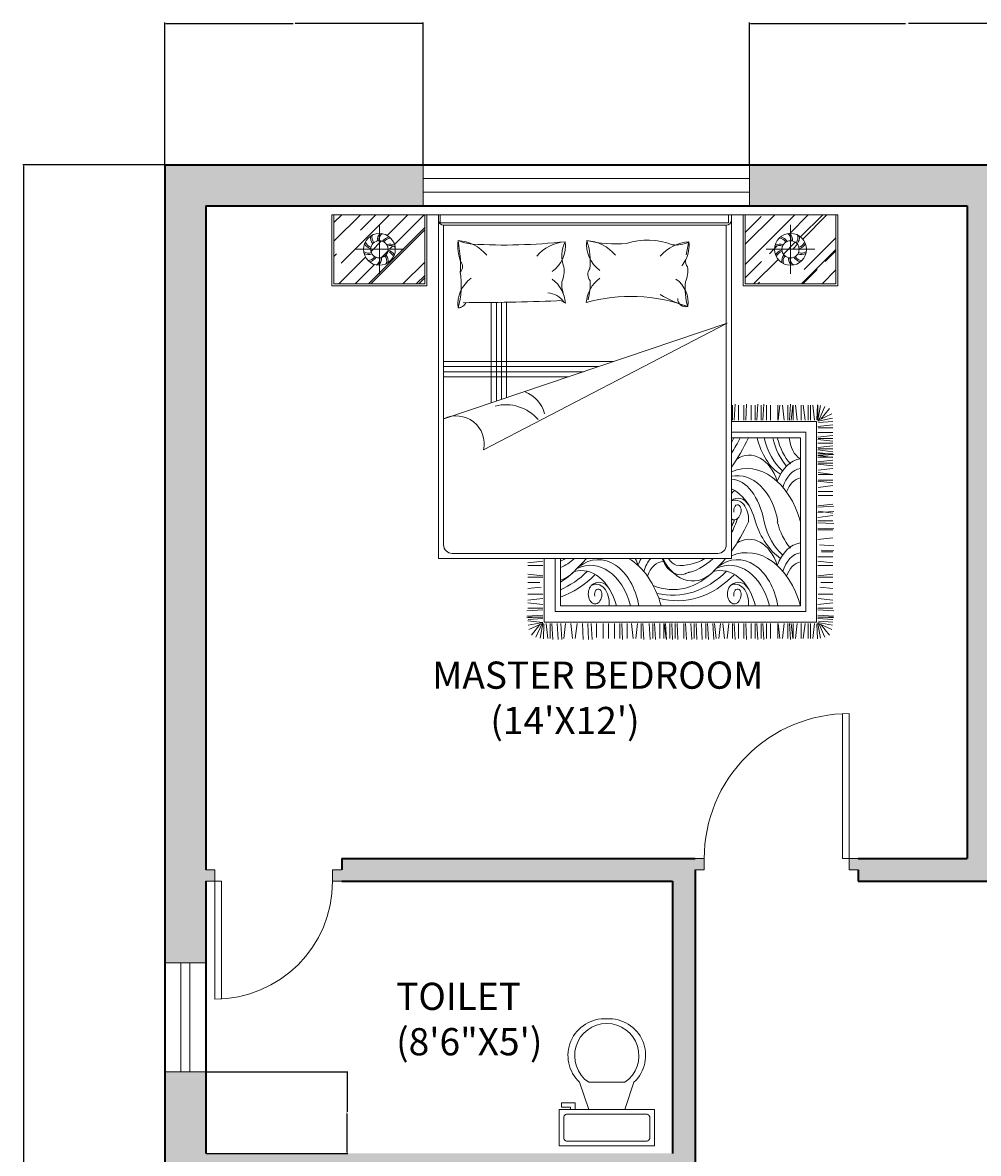
# Model space of a CAD drawing. Units: inches. Extents: x 2948 to 4025, y 2171 to 2966.
# Tile 3 of 6: x 2948 to 3159, y 2560 to 2809. Entities that reach past the tile are written whole.
import ezdxf

# ---------------------------------------------------------------- set-up
doc = ezdxf.new("R2010")
doc.units = ezdxf.units.IN
for name, color, linetype, lineweight in [('A-ANNO-DIMS', 2, 'Continuous', 18), ('A-AREA-IDEN', 7, 'Continuous', 18), ('A-DOOR', 3, 'Continuous', 18), ('A-FLOR-FIXT', 9, 'Continuous', 18), ('A-FURN', 8, 'Continuous', 18), ('A-GLAZ', 4, 'Continuous', 18), ('A-WALL', 7, 'Continuous', 35), ('A-WALL-PATT', 252, 'Continuous', 13)]:
    doc.layers.add(name, color=color, linetype=linetype, lineweight=lineweight)
doc.styles.get("Standard").update_dxf_attribs({"font": 'arial.ttf'})
doc.dimstyles.get("Standard").update_dxf_attribs({"dimtxt": 0.18, "dimasz": 0.18, "dimexe": 0.18, "dimexo": 0.0625, "dimgap": 0.09, "dimtad": 0, "dimtih": 1, "dimtoh": 1, "dimdec": 4, "dimzin": 0, "dimdsep": 46, "dimtxsty": 'Standard', "dimcen": 0.09, "dimadec": 0, "dimazin": 0, "dimtfac": 1, "dimtdec": 4, "dimtofl": 0, "dimtmove": 0, "dimatfit": 3, "dimfxl": 1, "dimtolj": 1, "dimtzin": 0, "dimarcsym": 0})

# ---------------------------------------------------------------- blocks, each defined once
blk = doc.blocks.new('A$C64B41DC1')
for p, q in [((0, 2.5079), (2.9903, 2.5079)), ((0, 2.0879), (0, 2.5079)), ((0.012, 2.4618), (0.0581, 2.5079)), ((0.012, 2.3515), (0.1684, 2.5079)), ((0.012, 2.0999), (0.012, 2.5079)), ((0.0543, 2.2213), (0.3409, 2.5079)), ((0.1689, 2.4179), (0.2589, 2.5079)), ((0.3265, 2.386), (0.4484, 2.5079)), ((0.3699, 2.3332), (0.5445, 2.5079)), ((0.548, 2.5079), (0.548, 2.0999)), ((0.56, 2.5079), (0.56, 2.0879)), ((0.6301, 2.5079), (0.6301, 0.4779)), ((0.6401, 2.461), (0.6401, 2.5079)), ((0.6401, 2.5079), (2.344, 2.5079)), ((2.344, 2.5079), (2.3601, 2.5079)), ((2.344, 2.5079), (2.344, 2.461)), ((2.3601, 2.5079), (2.3601, 2.4761)), ((2.3601, 0.4779), (2.3601, 2.5079)), ((2.4303, 2.5079), (2.4303, 2.0879)), ((2.4423, 2.5079), (2.4423, 2.0999)), ((2.4423, 2.3333), (2.6169, 2.5079)), ((2.4423, 2.2145), (2.7357, 2.5079)), ((2.4423, 2.404), (2.5354, 2.4971)), ((2.705, 2.398), (2.8149, 2.5079)), ((2.7691, 2.3772), (2.8998, 2.5079)), ((2.7819, 2.3646), (2.9252, 2.5079)), ((2.9783, 2.0999), (2.9783, 2.5079)), ((2.9903, 2.0879), (2.9903, 2.5079)), ((0.2157, 2.0999), (0.548, 2.4322)), ((0.2299, 2.0999), (0.548, 2.418)), ((0.2804, 2.1597), (0.2804, 2.4481)), ((2.344, 2.461), (0.6401, 2.461)), ((0.6601, 2.4461), (1.4951, 2.4461)), ((0.6601, 2.4461), (0.6601, 0.5579)), ((1.4951, 2.4461), (0.6697, 2.4461)), ((2.3301, 2.4461), (1.4951, 2.4461)), ((2.3301, 0.5579), (2.3301, 2.4461)), ((2.7099, 2.1597), (2.7099, 2.4481)), ((0.2311, 2.2906), (0.2937, 2.3532)), ((2.6674, 2.2756), (2.7382, 2.3464)), ((2.7914, 2.1846), (2.9783, 2.3715)), ((0.012, 2.261), (0.0275, 2.2765)), ((0.1362, 2.3039), (0.4246, 2.3039)), ((0.2905, 2.2539), (0.3304, 2.2938)), ((0.3405, 2.3039), (0.3605, 2.3238)), ((2.8541, 2.3039), (2.5657, 2.3039)), ((2.5849, 2.2779), (2.6158, 2.3088)), ((2.6158, 2.3088), (2.6313, 2.3243)), ((2.7249, 2.3076), (2.7512, 2.3339)), ((2.7746, 2.0999), (2.9783, 2.3036)), ((2.9144, 2.2312), (2.9783, 2.2951)), ((0.0404, 2.0999), (0.1982, 2.2578)), ((0.1365, 2.0999), (0.251, 2.2144)), ((0.4194, 2.0999), (0.548, 2.2285)), ((2.4423, 2.1353), (2.5382, 2.2312)), ((2.4918, 2.0999), (2.6366, 2.2447)), ((0.4986, 2.0999), (0.548, 2.1493)), ((2.7831, 2.0999), (2.8678, 2.1846)), ((2.8962, 2.0999), (2.9783, 2.182)), ((0.56, 2.0879), (0, 2.0879)), ((0.548, 2.0999), (0.012, 2.0999)), ((0.5127, 2.0999), (0.548, 2.1352)), ((2.4303, 2.0879), (2.9903, 2.0879)), ((2.4423, 2.0999), (2.9783, 2.0999)), ((2.5172, 2.0999), (2.5269, 2.1096)), ((0.9415, 1.9902), (0.9415, 1.3975)), ((0.9715, 1.9906), (0.9715, 1.4076)), ((1.0015, 1.991), (1.0015, 1.4177)), ((1.0315, 1.9916), (1.0315, 1.4279)), ((2.3349, 1.8678), (0.6613, 1.3029)), ((0.8956, 1.1191), (2.3349, 1.8678)), ((1.6636, 1.6412), (0.6601, 1.6412)), ((1.5748, 1.6112), (0.6601, 1.6112)), ((2.3665, 1.295), (2.3665, 1.3839)), ((2.377, 1.295), (2.3822, 1.3891)), ((2.4032, 1.295), (2.4032, 1.3839)), ((2.4346, 1.295), (2.4346, 1.3839)), ((2.4451, 1.295), (2.4503, 1.3891)), ((2.4774, 1.2957), (2.4774, 1.3837)), ((2.5, 1.295), (2.5, 1.3839)), ((2.5105, 1.295), (2.5157, 1.3891)), ((2.5367, 1.295), (2.5367, 1.3839)), ((2.5471, 1.295), (2.5524, 1.3891)), ((2.5681, 1.295), (2.5681, 1.3839)), ((2.5918, 1.295), (2.5918, 1.3839)), ((2.6346, 1.2957), (2.6346, 1.3837)), ((2.6362, 1.2957), (2.6467, 1.3839)), ((2.6729, 1.295), (2.6624, 1.3839)), ((2.6938, 1.295), (2.6938, 1.3839)), ((2.7043, 1.295), (2.7095, 1.3891)), ((2.7127, 1.2957), (2.7232, 1.3839)), ((2.7253, 1.295), (2.7253, 1.3839)), ((2.7494, 1.295), (2.7389, 1.3839)), ((2.7718, 1.295), (2.7718, 1.3839)), ((2.7959, 1.295), (2.7854, 1.3839)), ((2.8146, 1.2957), (2.8146, 1.3837)), ((2.8146, 1.2957), (2.8146, 1.3837)), ((2.8282, 1.295), (2.8282, 1.3839)), ((2.8282, 1.295), (2.8282, 1.3839)), ((2.8523, 1.295), (2.8418, 1.3839)), ((2.8523, 1.295), (2.8418, 1.3839)), ((2.8653, 1.2966), (2.8688, 1.3861)), ((2.8711, 1.2957), (2.8711, 1.3837)), ((2.8711, 1.2957), (2.8875, 1.3822)), ((2.8765, 1.2958), (2.9132, 1.3758)), ((2.8893, 1.3011), (2.9394, 1.3636)), ((2.3601, 1.2873), (2.8639, 1.2873)), ((2.8639, 1.2873), (2.8639, 0.1018)), ((2.8713, 1.2927), (2.954, 1.3315)), ((2.8717, 1.2884), (2.9588, 1.3058)), ((2.8744, 1.2817), (2.9603, 1.2869)), ((2.3601, 1.2233), (2.7999, 1.2233)), ((2.7999, 1.2233), (2.7999, 0.1658)), ((2.8716, 1.2565), (2.9605, 1.2669)), ((2.8716, 1.2212), (2.9605, 1.2212)), ((2.8716, 1.1947), (2.9605, 1.2052)), ((2.8723, 1.2489), (2.9603, 1.2489)), ((2.3601, 1.1913), (2.7679, 1.1912)), ((2.7679, 1.1912), (2.7679, 0.1978)), ((2.8716, 1.181), (2.9605, 1.1705)), ((2.8716, 1.1595), (2.9605, 1.1595)), ((2.8716, 1.133), (2.9605, 1.1435)), ((2.8723, 1.1872), (2.9603, 1.1872)), ((2.8716, 1.1193), (2.9605, 1.1088)), ((2.8716, 1.1035), (2.9605, 1.093)), ((2.8716, 1.0965), (2.9605, 1.0965)), ((2.8716, 1.086), (2.9657, 1.0913)), ((2.8716, 1.0756), (2.9605, 1.0756)), ((2.8723, 1.1255), (2.9603, 1.1255)), ((2.8723, 1.0858), (2.9605, 1.0753)), ((2.8716, 1.0491), (2.9605, 1.0596)), ((2.8716, 1.0354), (2.9605, 1.0249)), ((2.8723, 1.0416), (2.9603, 1.0416)), ((2.8723, 0.9987), (2.9605, 1.0092)), ((2.8723, 0.985), (2.9605, 0.9745)), ((2.8723, 0.9735), (2.9603, 0.9735)), ((2.8723, 0.9408), (2.9603, 0.9408)), ((2.8716, 0.9346), (2.9605, 0.9241)), ((2.8723, 0.8979), (2.9605, 0.9084)), ((2.8723, 0.8726), (2.9603, 0.8726)), ((2.8723, 0.8505), (2.9603, 0.8505)), ((2.8716, 0.7885), (2.9605, 0.799)), ((2.8716, 0.7818), (2.9657, 0.787)), ((2.8716, 0.7503), (2.9657, 0.7556)), ((2.8723, 0.7571), (2.9605, 0.7466)), ((2.8716, 0.7204), (2.9605, 0.7309)), ((2.8716, 0.6995), (2.9605, 0.6995)), ((2.8716, 0.689), (2.9657, 0.6838)), ((2.8716, 0.6576), (2.9657, 0.6523)), ((2.8716, 0.6471), (2.9605, 0.6471)), ((2.8716, 0.5903), (2.9605, 0.6007)), ((2.882, 0.5582), (2.9657, 0.5536)), ((0.6301, 0.4779), (2.3601, 0.4779)), ((0.7101, 0.5079), (2.2801, 0.5079)), ((1.2542, 0.1018), (1.2542, 0.4779)), ((1.3182, 0.1658), (1.3182, 0.4779)), ((1.3502, 0.1978), (1.3502, 0.4779)), ((2.8716, 0.4877), (2.9603, 0.4877)), ((2.8909, 0.5263), (2.9657, 0.5222)), ((2.8928, 0.5169), (2.9605, 0.5169)), ((1.2465, 0.4625), (1.1576, 0.452)), ((1.2465, 0.4365), (1.1577, 0.4365)), ((2.8716, 0.4625), (2.9605, 0.452)), ((2.8716, 0.4365), (2.9603, 0.4365)), ((1.2465, 0.3746), (1.1576, 0.3851)), ((1.2465, 0.3684), (1.1577, 0.3684)), ((1.2285, 0.3357), (1.1577, 0.3357)), ((2.8716, 0.3746), (2.9605, 0.3851)), ((2.8716, 0.3684), (2.9603, 0.3684)), ((2.8896, 0.3357), (2.9603, 0.3357)), ((1.2355, 0.3092), (1.1576, 0.3)), ((1.2457, 0.2676), (1.1577, 0.2676)), ((2.8723, 0.2676), (2.9603, 0.2676)), ((2.8826, 0.3092), (2.9605, 0.3)), ((1.2457, 0.2423), (1.1576, 0.2319)), ((1.2465, 0.2057), (1.1576, 0.2161)), ((2.8716, 0.2057), (2.9605, 0.2161)), ((2.8723, 0.2423), (2.9605, 0.2319)), ((1.2465, 0.1742), (1.1524, 0.169)), ((1.2465, 0.1428), (1.1524, 0.1376)), ((1.2465, 0.1847), (1.1576, 0.1847)), ((2.7999, 0.1658), (1.3182, 0.1658)), ((2.7679, 0.1978), (1.3502, 0.1978)), ((2.8716, 0.1847), (2.9605, 0.1847)), ((2.8716, 0.1742), (2.9657, 0.169)), ((2.8716, 0.1428), (2.9657, 0.1376)), ((1.2465, 0.1334), (1.1524, 0.1281)), ((1.2465, 0.1323), (1.1576, 0.1323)), ((1.2465, 0.1323), (1.1576, 0.1323)), ((1.2465, 0.1), (1.1576, 0.1105)), ((1.2465, 0.1229), (1.1588, 0.1168)), ((1.2464, 0.1007), (1.1592, 0.0833)), ((1.2468, 0.0964), (1.1641, 0.0576)), ((1.2288, 0.088), (1.1787, 0.0255)), ((1.2415, 0.0933), (1.2049, 0.0133)), ((1.247, 0.0934), (1.2306, 0.0069)), ((1.2527, 0.0925), (1.2493, 0.003)), ((2.8639, 0.1018), (1.2542, 0.1018)), ((1.2658, 0.0941), (1.2762, 0.0052)), ((1.2899, 0.0941), (1.2899, 0.0052)), ((1.2999, 0.0941), (1.3051, 0)), ((1.3313, 0.0941), (1.3365, 0)), ((1.3523, 0.0941), (1.3575, 0)), ((1.3804, 0.0941), (1.3699, 0.0052)), ((1.4119, 0.0934), (1.4223, 0.0052)), ((1.4485, 0.0941), (1.438, 0.0052)), ((1.48, 0.0941), (1.4852, 0)), ((1.5114, 0.0941), (1.5166, 0)), ((1.5323, 0.0941), (1.5376, 0)), ((1.5638, 0.0941), (1.5638, 0.0105)), ((1.6021, 0.0941), (1.6021, 0.0052)), ((1.6336, 0.0941), (1.6336, 0.0052)), ((1.6702, 0.0941), (1.6702, 0.0052)), ((1.7017, 0.0941), (1.7017, 0.0052)), ((1.7122, 0.0941), (1.7174, 0)), ((1.7445, 0.0934), (1.7445, 0.0054)), ((1.7698, 0.0934), (1.7803, 0.0052)), ((1.8065, 0.0941), (1.796, 0.0052)), ((1.8274, 0.0941), (1.8274, 0.0052)), ((1.8379, 0.0941), (1.8431, 0)), ((1.8746, 0.0941), (1.8798, 0)), ((1.8955, 0.0941), (1.8955, 0.0052)), ((1.906, 0.0941), (1.9113, 0)), ((1.9384, 0.0934), (1.9384, 0.0054)), ((1.9609, 0.0941), (1.9609, 0.0052)), ((1.9636, 0.0934), (1.9741, 0.0052)), ((1.9714, 0.0941), (1.9766, 0)), ((1.9976, 0.0941), (1.9976, 0.0052)), ((2.0081, 0.0941), (2.0133, 0)), ((2.029, 0.0941), (2.029, 0.0052)), ((2.0395, 0.0941), (2.0447, 0)), ((2.0797, 0.0941), (2.0797, 0.0052)), ((2.0902, 0.0941), (2.0954, 0)), ((2.1216, 0.0941), (2.1269, 0)), ((2.1412, 0.0941), (2.1412, 0.0052)), ((2.1517, 0.0941), (2.1569, 0)), ((2.1831, 0.0941), (2.1884, 0)), ((2.2093, 0.0941), (2.2093, 0.0052)), ((2.2198, 0.0941), (2.225, 0)), ((2.2512, 0.0941), (2.2565, 0)), ((2.2603, 0.0934), (2.2707, 0.0052)), ((2.2969, 0.0941), (2.2864, 0.0052)), ((2.3089, 0.0934), (2.3193, 0.0052)), ((2.3455, 0.0941), (2.3351, 0.0052)), ((2.3665, 0.0941), (2.3665, 0.0052)), ((2.377, 0.0941), (2.3822, 0)), ((2.4032, 0.0941), (2.4032, 0.0052)), ((2.4346, 0.0941), (2.4346, 0.0052)), ((2.4451, 0.0941), (2.4503, 0)), ((2.4774, 0.0934), (2.4774, 0.0054)), ((2.5, 0.0941), (2.5, 0.0052)), ((2.5105, 0.0941), (2.5157, 0)), ((2.5367, 0.0941), (2.5367, 0.0052)), ((2.5471, 0.0941), (2.5524, 0)), ((2.5681, 0.0941), (2.5681, 0.0052)), ((2.5918, 0.0941), (2.5918, 0.0052)), ((2.6346, 0.0934), (2.6346, 0.0054)), ((2.6362, 0.0934), (2.6467, 0.0052)), ((2.6729, 0.0941), (2.6624, 0.0052)), ((2.6938, 0.0941), (2.6938, 0.0052)), ((2.7043, 0.0941), (2.7095, 0)), ((2.7127, 0.0934), (2.7232, 0.0052)), ((2.7253, 0.0941), (2.7253, 0.0052)), ((2.7494, 0.0941), (2.7389, 0.0052)), ((2.7718, 0.0941), (2.7718, 0.0052)), ((2.7959, 0.0941), (2.7854, 0.0052)), ((2.8146, 0.0934), (2.8146, 0.0054)), ((2.8282, 0.0941), (2.8282, 0.0052)), ((2.8523, 0.0941), (2.8418, 0.0052)), ((2.8653, 0.0925), (2.8688, 0.003)), ((2.8711, 0.0934), (2.8875, 0.0069)), ((2.8713, 0.0964), (2.954, 0.0576)), ((2.8716, 0.1334), (2.9657, 0.1281)), ((2.8716, 0.1323), (2.9605, 0.1323)), ((2.8716, 0.1229), (2.9593, 0.1168)), ((2.8717, 0.1007), (2.9588, 0.0833)), ((2.8744, 0.1074), (2.9603, 0.1022)), ((2.8765, 0.0933), (2.9132, 0.0133)), ((2.8893, 0.088), (2.9394, 0.0255))]:
    blk.add_line(p, q)
at = {"ltscale": 10}
for p, q in [((1.4859, 1.5812), (0.6601, 1.5812)), ((1.397, 1.5512), (0.6601, 1.5512))]:
    blk.add_line(p, q, dxfattribs=at)
for centre, radius in [((0.2804, 2.3039), 0.0942), ((0.2804, 2.3039), 0.051), ((2.7099, 2.3039), 0.0942), ((2.7099, 2.3039), 0.051)]:
    blk.add_circle(centre, radius)
for centre, radius, start, end in [((0.6601, 2.4761), 0.03, 180, 270), ((2.3301, 2.4761), 0.03, 270, 0), ((0.2417, 2.3614), 0.0462, 196.30017, 256.53802), ((0.2887, 2.3745), 0.0605, 172.17003, 218.48975), ((0.2828, 2.3731), 0.0462, 160.30017, 220.53802), ((0.3286, 2.3561), 0.0605, 136.17003, 182.48975), ((0.3231, 2.3585), 0.0462, 124.30017, 184.53802), ((0.3501, 2.3178), 0.0605, 100.17003, 146.48975), ((0.347, 2.323), 0.0462, 88.30017, 148.53802), ((1.0526, 2.3302), 0.3085, 175.30484, 198.69419), ((-0.8702, 2.0941), 1.6364, 4.80985, 9.18918), ((0.8579, 2.6278), 0.2948, 247.51785, 264.26696), ((0.728, 2.111), 0.245, 40.4189, 85.9871), ((1.0164, 5.7096), 3.3803, 266.81337, 276.16021), ((1.3963, 2.1044), 0.245, 94.0129, 139.5811), ((1.1858, 2.3288), 0.1943, 306.5711, 5.88998), ((1.5348, 2.2652), 0.1767, 151.77364, 201.69827), ((1.6986, 2.3355), 0.1943, 174.11002, 233.4289), ((1.1481, 2.2311), 0.3783, 353.49469, 19.18669), ((1.6871, 3.192), 0.8561, 257.74383, 273.62843), ((1.4882, 2.111), 0.245, 40.4189, 85.9871), ((1.8674, 1.9709), 0.3878, 68.20259, 108.9817), ((2.1269, 2.1044), 0.245, 94.0129, 139.5811), ((2.0342, 2.4856), 0.1563, 261.59582, 298.90918), ((1.9165, 2.3288), 0.1943, 333.73715, 5.88998), ((2.6058, 2.2028), 0.517, 163.60457, 172.3273), ((2.6433, 2.323), 0.0462, 31.46198, 91.69983), ((2.6402, 2.3178), 0.0605, 33.51025, 79.82997), ((2.6672, 2.3585), 0.0462, 355.46198, 55.69983), ((2.6617, 2.3561), 0.0605, 357.51025, 43.82997), ((2.7075, 2.3731), 0.0462, 319.46198, 19.69983), ((2.7016, 2.3745), 0.0605, 321.51025, 7.82997), ((2.7486, 2.3614), 0.0462, 283.46198, 343.69983), ((0.2153, 2.3276), 0.0462, 232.30017, 292.53802), ((0.2158, 2.3336), 0.0605, 244.17003, 290.48975), ((0.2457, 2.3659), 0.0605, 208.17003, 254.48975), ((0.272, 2.2333), 0.0605, 352.17003, 38.48975), ((0.3449, 2.2742), 0.0605, 64.17003, 110.48975), ((0.3455, 2.2802), 0.0462, 52.30017, 112.53802), ((0.3191, 2.2464), 0.0462, 16.30017, 76.53802), ((0.3151, 2.2419), 0.0605, 28.17003, 74.48975), ((2.6448, 2.2802), 0.0462, 67.46198, 127.69983), ((2.6454, 2.2742), 0.0605, 69.51025, 115.82997), ((2.6752, 2.2419), 0.0605, 105.51025, 151.82997), ((2.6712, 2.2464), 0.0462, 103.46198, 163.69983), ((2.7182, 2.2333), 0.0605, 141.51025, 187.82997), ((2.7744, 2.3336), 0.0605, 249.51025, 295.82997), ((2.775, 2.3276), 0.0462, 247.46198, 307.69983), ((2.7446, 2.3659), 0.0605, 285.51025, 331.82997), ((0.2138, 2.2848), 0.0462, 268.30017, 328.53802), ((0.2107, 2.29), 0.0605, 280.17003, 326.48975), ((0.2377, 2.2493), 0.0462, 304.30017, 4.53802), ((0.2322, 2.2517), 0.0605, 316.17003, 2.48975), ((0.2779, 2.2347), 0.0462, 340.30017, 40.53802), ((0.7274, 2.2013), 0.0446, 314.4736, 42.17134), ((-1.6008, 2.277), 2.3618, 357.39054, 358.88764), ((1.9165, 2.3288), 0.1943, 320.94042, 333.73715), ((2.1347, 2.2313), 0.0459, 165.35061, 223.26844), ((2.7123, 2.2347), 0.0462, 139.46198, 199.69983), ((2.7581, 2.2517), 0.0605, 177.51025, 223.82997), ((2.7526, 2.2493), 0.0462, 175.46198, 235.69983), ((2.7796, 2.29), 0.0605, 213.51025, 259.82997), ((2.7765, 2.2848), 0.0462, 211.46198, 271.69983), ((0.2688, 2.0945), 0.4956, 344.0243, 8.70709), ((1.204, 2.1778), 0.1681, 337.01697, 7.53676), ((1.5671, 2.1546), 0.0547, 142.08329, 220.902), ((1.9346, 2.1778), 0.1681, 337.01697, 7.53676), ((0.9385, 1.978), 0.1943, 126.5711, 185.88998), ((1.1858, 1.9714), 0.1943, 4.31813, 53.4289), ((1.5415, 2.0969), 0.1834, 175.22328, 196.23004), ((1.7059, 1.9714), 0.204, 127.11975, 175.09005), ((1.1965, 2.0983), 0.3299, 343.79543, 3.55541), ((1.9394, 1.991), 0.1651, 351.26213, 55.75721), ((2.4617, 2.0719), 0.3745, 173.82958, 196.4356), ((1.2687, 1.9248), 0.1223, 33.62799, 86.47438), ((1.7676, 1.0629), 0.9631, 69.65065, 105.96307), ((2.2748, 2.5795), 0.6373, 238.34989, 254.31375), ((2.0911, 2.0123), 0.0478, 179.77267, 283.80184), ((0.7417, 2.0149), 0.057, 273.47085, 328.54118), ((0.728, 2.2025), 0.245, 274.0129, 278.34166), ((0.7246, 18.8439), 16.8552, 270.17399, 272.05214), ((1.3401, 1.9404), 0.0603, 49.09906, 101.37023), ((1.0747, 1.2871), 0.1871, 14.1863, 69.12121), ((1.0274, 1.1334), 0.2527, 40.62904, 104.37123), ((0.7347, 1.1553), 0.1649, 347.31088, 116.44537), ((0.7101, 0.5579), 0.05, 180, 270), ((2.2801, 0.5579), 0.05, 270, 0)]:
    blk.add_arc(centre, radius, start, end)
for centre, major_axis, ratio, start_param, end_param in [((1.9938, 1.6262), (0, -0.7531), 0.68, 0.797284, 0.954936), ((2.0643, 1.466), (0, -0.5322), 0.68, 7.239912, 7.311536), ((1.9052, 1.7397), (0, -0.9842), 0.68, 0.74745, 0.979724), ((2.7455, 1.3081), (0, 0.3614), 0.68, 1.900046, 2.742661), ((2.7868, 1.3081), (0, 0.3614), 0.68, 1.900046, 2.614747), ((2.8372, 1.3081), (0, 0.3614), 0.68, 1.900046, 2.479658), ((2.8607, 1.3211), (0, 0.3614), 0.68, 1.938265, 2.479658), ((2.8057, 1.2079), (0, -0.1524), 0.68, 4.821745, 5.895886), ((2.4665, 0.8216), (0, -0.2664), 0.68, 2.006169, 3.565187), ((2.4513, 0.5069), (0, 0.502), 0.68, 5.095327, 6.553458), ((2.7862, 0.8069), (0, -0.2615), 0.68, 3.244645, 4.205018), ((2.7784, 0.8289), (0, -0.1802), 0.68, 3.227058, 4.318474), ((2.396, 0.6032), (0, 0.3641), 0.68, -1.3172, 0.145284), ((2.3507, 0.5642), (0.0073, 0.3819), 0.56205, -1.21172, -0.009991), ((2.7821, 0.7971), (0, -0.1589), 0.68, 3.272942, 4.229533), ((2.2964, 0.5771), (0, -0.3263), 0.68, 1.938944, 2.850232), ((2.0403, 1.6015), (0, -0.8763), 0.68, 6.849801, 6.887077), ((2.4005, 0.7132), (0, -0.1214), 0.68, 2.284368, 3.652258), ((2.3834, 0.7081), (0, 0.1147), 0.68, 4.593909, 6.585576), ((2.3774, 0.7653), (0, -0.0593), 0.68, 5.841311, 7.755362), ((2.3961, 0.7628), (0, -0.0317), 0.68, 1.462497, 5.046281), ((1.9938, 1.1295), (-0.0678, 0.7439), 0.610498, 3.917146, 4.063997), ((2.0643, 0.9693), (0, -0.5322), 0.68, 7.239912, 7.336618), ((1.9052, 1.243), (0, -0.9842), 0.68, 0.74745, 0.979724), ((2.7455, 0.8114), (-0.0599, 0.3735), 0.695517, 1.775813, 2.548612), ((2.7868, 0.8114), (0, 0.3614), 0.68, 1.900046, 2.614747), ((2.8607, 0.8243), (0, 0.3614), 0.68, 1.938265, 2.479658), ((2.4665, 0.3249), (0, -0.2664), 0.68, 2.006169, 3.565187), ((2.4513, 0.0102), (0, 0.502), 0.68, 5.095327, 6.553458), ((2.7862, 0.3102), (0, -0.2615), 0.68, 3.244645, 4.205018), ((1.242, 0.9693), (0, -0.5322), 0.68, 6.586764, 6.677612), ((1.1714, 1.1295), (-0.1157, 0.7241), 0.59432, 3.291697, 3.50733), ((1.0828, 1.243), (0, -0.9842), 0.68, 0.565948, 0.680366), ((1.5283, 0.0674), (0, -0.3703), 0.68, 1.930561, 3.464283), ((1.5736, 0.1065), (0, 0.3641), 0.68, -1.3172, 0.476403), ((1.6289, 0.0102), (0, 0.502), 0.68, 6.655152, 6.661293), ((1.6289, 0.0102), (0, 0.502), 0.68, 5.095327, 5.911219), ((1.6442, 0.3249), (0, -0.2664), 0.68, 2.006169, 2.182797), ((1.9638, 0.3102), (0, -0.2615), 0.68, 4.015924, 4.205018), ((1.956, 0.3322), (0, -0.1802), 0.68, 3.770744, 4.318474), ((2.0606, 0.5616), (0, -0.1803), 0.68, 5.194792, 5.929328), ((2.0606, 0.5616), (0, -0.1803), 0.68, 5.194792, 6.723255), ((2.1315, 0.6603), (0, -0.3155), 0.68, 5.328638, 6.949396), ((2.0549, 0.5656), (0, -0.1303), 0.68, 5.450951, 6.054641), ((2.0643, 0.9693), (0, -0.5322), 0.68, 6.20013, 6.677612), ((1.9938, 1.1295), (-0.0678, 0.7439), 0.610498, 3.199135, 3.592282), ((1.9052, 1.243), (0, -0.9842), 0.68, 0.565948, 0.680366), ((2.3507, 0.0674), (0, -0.3703), 0.68, 1.930561, 3.464283), ((2.396, 0.1065), (0, 0.3641), 0.68, -1.3172, 0.476403), ((2.4513, 0.0102), (0, 0.502), 0.68, 6.655152, 6.661293), ((2.7784, 0.3322), (0, -0.1802), 0.68, 3.227058, 4.318474), ((1.1933, 0.9181), (0, -0.624), 0.68, 0.378672, 0.625379), ((1.3091, 0.6603), (0, -0.3155), 0.68, 6.475719, 6.949396), ((1.1911, 1.1066), (0, 0.8458), 0.68, 3.421828, 3.728616), ((1.474, 0.0804), (0, -0.3263), 0.68, 1.938944, 3.339184), ((1.9597, 0.3004), (0, -0.1589), 0.68, 3.14258, 4.229533), ((2.0157, 0.9181), (0, -0.624), 0.68, -0.280078, 0.625379), ((2.0135, 1.1066), (0, 0.8458), 0.68, 2.978727, 3.728616), ((2.2964, 0.0804), (0, -0.3263), 0.68, 1.938944, 3.339184), ((2.7821, 0.3004), (0, -0.1589), 0.68, 3.272942, 4.229533), ((1.2179, 1.1047), (0, -0.8763), 0.68, 6.507006, 6.887077), ((1.5781, 0.2165), (0, -0.1214), 0.68, 2.284368, 3.726131), ((2.0403, 1.1047), (0, -0.8763), 0.68, 6.099302, 6.887077), ((2.4005, 0.2165), (0, -0.1214), 0.68, 2.284368, 3.726131), ((1.555, 0.2685), (0, -0.0593), 0.68, 3.732151, 7.755362), ((1.561, 0.2114), (0, 0.1147), 0.68, 4.593909, 6.647252), ((1.5737, 0.2661), (0, -0.0317), 0.68, 1.462497, 5.046281), ((2.3774, 0.2685), (0, -0.0593), 0.68, 3.732151, 7.755362), ((2.3834, 0.2114), (0, 0.1147), 0.68, 4.593909, 6.647252), ((2.3961, 0.2661), (0, -0.0317), 0.68, 1.462497, 5.046281)]:
    blk.add_ellipse(centre, major_axis=major_axis, ratio=ratio, start_param=start_param, end_param=end_param)
blk = doc.blocks.new('*U8')
for p, q in [((9.5, -6), (9.5, -2)), ((-10, -8.5), (-8, -8.5)), ((-10, -9.5), (-10, -8.5)), ((-7, -9.5), (-10, -9.5)), ((-8, -8.5), (-8, -8)), ((-7, -8), (-7, -9.5)), ((-4, -8), (-6, -14)), ((4, -8), (6, -14)), ((4, -14), (-4, -14))]:
    blk.add_line(p, q)
blk.add_lwpolyline([(10.5, -8), (10.5, 0), (-10.5, 0), (-10.5, -8)], close=True)
for points in [[(-9.5, -2), (-9.5, -6)], [(8.5, -1), (-8.5, -1)], [(-8.5, -7), (8.5, -7)]]:
    blk.add_lwpolyline(points)
for centre, radius, start, end in [((-8.625, -1.875), 0.8839, 81.8699, 188.1301), ((8.625, -1.875), 0.8839, 351.8699, 98.1301), ((-8.625, -6.125), 0.8839, 171.869898, 278.1301), ((8.625, -6.125), 0.8839, 261.8699, 8.1301), ((-0.4772, -19.9188), 8.0953, 133.01722, 273.38), ((0.0374, -19.8731), 7.127, 124.50543, 269.7), ((-0.0373, -19.8731), 7.127, 270.3, 55.4946), ((0.4773, -19.9188), 8.0953, 266.62, 46.9828)]:
    blk.add_arc(centre, radius, start, end)
blk = doc.blocks.new('DOOR-SWING-32IN')
for p, q in [((2, 34.5), (0, 34.5)), ((2, 32), (2, 34.5)), ((34, 32), (34, 34.5)), ((34, 34.5), (36, 34.5)), ((0, 32), (2, 32)), ((2, 32), (2, 0)), ((2, 32), (3.5, 32)), ((3.5, 32), (3.5, 0.04)), ((36, 32), (34, 32))]:
    blk.add_line(p, q)
blk.add_arc((2, 32), 32, 270, 0)
blk = doc.blocks.new('DOOR-SWING-26IN')
for p, q in [((26, 30), (26, 28)), ((28.5, 28), (28.5, 30)), ((26, 28), (28.5, 28)), ((26, 3.5), (0.04, 3.5)), ((26, 3.5), (26, 2)), ((26, 2), (0, 2)), ((26, 0), (26, 2)), ((26, 2), (28.5, 2)), ((28.5, 2), (28.5, 0))]:
    blk.add_line(p, q)
blk.add_arc((26, 2), 26, 90, 180)
blk = doc.blocks.new('WIN-72IN')
for p, q in [((0, 0), (0, 9)), ((72, 0), (72, 9)), ((72, 6), (0, 6)), ((72, 3), (0, 3))]:
    blk.add_line(p, q)
blk = doc.blocks.new('WIN-24IN')
for p, q in [((0, 0), (0, 9)), ((24, 0), (24, 9)), ((24, 5.5), (0, 5.5)), ((24, 3.5), (0, 3.5))]:
    blk.add_line(p, q)
blk = doc.blocks.new('*D38')
at = {"layer": 'A-ANNO-DIMS', "color": 0, "lineweight": -2, "transparency": 16777216}
for p, q in [((2979.45, 2777.99), (2948.13, 2777.99)), ((2948.31, 2777.81), (2948.31, 2507.17)), ((2948.31, 2236.17), (2948.31, 2506.8)), ((3217.45, 2235.99), (2948.13, 2235.99))]:
    blk.add_line(p, q, dxfattribs=at)
at = {"layer": 'A-ANNO-DIMS', "color": 0, "transparency": 16777216}
for points in [[(2948.28, 2777.81), (2948.34, 2777.81), (2948.31, 2777.99)], [(2948.28, 2236.17), (2948.34, 2236.17), (2948.31, 2235.99)]]:
    blk.add_solid(points, dxfattribs=at)
at = {"layer": 'Defpoints', "color": 0, "transparency": 16777216}
for p in [(2948.31, 2777.99), (2979.51, 2777.99), (3217.51, 2235.99)]:
    blk.add_point(p, dxfattribs=at)
at = {"layer": 'A-ANNO-DIMS', "color": 0, "transparency": 16777216, "insert": (2948.31, 2506.99), "char_height": 0.18, "attachment_point": 5}
blk.add_mtext('\\A1;542', dxfattribs=at)
blk = doc.blocks.new('*D39')
at = {"layer": 'A-ANNO-DIMS', "color": 0, "lineweight": -2, "transparency": 16777216}
for p, q in [((2979.51, 2778.05), (2979.51, 2809.37)), ((2979.69, 2809.19), (3007.79, 2809.19)), ((3036.33, 2809.19), (3008.23, 2809.19)), ((3036.51, 2778.05), (3036.51, 2809.37))]:
    blk.add_line(p, q, dxfattribs=at)
at = {"layer": 'A-ANNO-DIMS', "color": 0, "transparency": 16777216}
for points in [[(2979.69, 2809.22), (2979.69, 2809.16), (2979.51, 2809.19)], [(3036.33, 2809.22), (3036.33, 2809.16), (3036.51, 2809.19)]]:
    blk.add_solid(points, dxfattribs=at)
at = {"layer": 'Defpoints', "color": 0, "transparency": 16777216}
for p in [(3036.51, 2809.19), (2979.51, 2777.99), (3036.51, 2777.99)]:
    blk.add_point(p, dxfattribs=at)
at = {"layer": 'A-ANNO-DIMS', "color": 0, "transparency": 16777216, "insert": (3008.01, 2809.19), "char_height": 0.18, "attachment_point": 5}
blk.add_mtext('\\A1;57', dxfattribs=at)
blk = doc.blocks.new('*D40')
at = {"layer": 'A-ANNO-DIMS', "color": 0, "lineweight": -2, "transparency": 16777216}
for p, q in [((3108.51, 2778.05), (3108.51, 2809.37)), ((3108.69, 2809.19), (3142.94, 2809.19)), ((3177.83, 2809.19), (3143.59, 2809.19)), ((3178.01, 2778.05), (3178.01, 2809.37))]:
    blk.add_line(p, q, dxfattribs=at)
at = {"layer": 'A-ANNO-DIMS', "color": 0, "transparency": 16777216}
for points in [[(3108.69, 2809.22), (3108.69, 2809.16), (3108.51, 2809.19)], [(3177.83, 2809.22), (3177.83, 2809.16), (3178.01, 2809.19)]]:
    blk.add_solid(points, dxfattribs=at)
at = {"layer": 'Defpoints', "color": 0, "transparency": 16777216}
for p in [(3178.01, 2809.19), (3108.51, 2777.99), (3178.01, 2777.99)]:
    blk.add_point(p, dxfattribs=at)
at = {"layer": 'A-ANNO-DIMS', "color": 0, "transparency": 16777216, "insert": (3143.26, 2809.19), "char_height": 0.18, "attachment_point": 5}
blk.add_mtext('\\A1;69.5', dxfattribs=at)
blk = doc.blocks.new('*D42')
at = {"layer": 'A-ANNO-DIMS', "color": 0, "lineweight": -2, "transparency": 16777216}
for p, q in [((2988.58, 2577.99), (3019.89, 2577.99)), ((3019.71, 2577.81), (3019.71, 2569.17)), ((3019.71, 2560.17), (3019.71, 2568.8)), ((2988.58, 2559.99), (3019.89, 2559.99))]:
    blk.add_line(p, q, dxfattribs=at)
at = {"layer": 'A-ANNO-DIMS', "color": 0, "transparency": 16777216}
for points in [[(3019.68, 2577.81), (3019.74, 2577.81), (3019.71, 2577.99)], [(3019.68, 2560.17), (3019.74, 2560.17), (3019.71, 2559.99)]]:
    blk.add_solid(points, dxfattribs=at)
at = {"layer": 'Defpoints', "color": 0, "transparency": 16777216}
for p in [(2988.51, 2577.99), (2988.51, 2559.99), (3019.71, 2559.99)]:
    blk.add_point(p, dxfattribs=at)
at = {"layer": 'A-ANNO-DIMS', "color": 0, "transparency": 16777216, "insert": (3019.71, 2568.99), "char_height": 0.18, "attachment_point": 5}
blk.add_mtext('\\A1;18', dxfattribs=at)

msp = doc.modelspace()

# ---------------------------------------------------------------- hatches: boundary and pattern name
at = {"layer": 'A-WALL-PATT'}
h = msp.add_hatch(color=256, dxfattribs=at)
h.dxf.hatch_style = 1
h.paths.add_polyline_path([(2988.5136, 2768.9862), (3036.5136, 2768.9862), (3036.5136, 2777.9862), (2979.5136, 2777.9862), (2979.5136, 2601.9862), (2988.5136, 2601.9862), (2988.5136, 2619.9862), (2990.5136, 2619.9862), (2990.5136, 2622.4862), (2988.5136, 2622.4862)])
h = msp.add_hatch(color=256, dxfattribs=at)
h.dxf.hatch_style = 1
h.paths.add_polyline_path([(3178.0136, 2777.9862), (3108.5136, 2777.9862), (3108.5136, 2768.9862), (3156.5136, 2768.9862), (3156.5136, 2624.9862), (3132.5136, 2624.9862), (3130.5136, 2624.9862), (3130.5136, 2622.4862), (3132.5136, 2622.4862), (3132.5136, 2619.9862), (3161.5136, 2619.9862), (3161.5136, 2667.9862), (3218.5136, 2667.9862), (3218.5136, 2660.9862), (3218.5136, 2658.9862), (3221.0136, 2658.9862), (3221.0136, 2660.9862), (3223.5136, 2660.9862), (3223.5136, 2676.9862), (3221.0136, 2676.9862), (3221.0136, 2678.9862), (3218.5136, 2678.9862), (3218.5136, 2676.9862), (3218.5136, 2672.9862), (3161.5136, 2672.9862), (3161.5136, 2768.9862), (3178.0136, 2768.9862)])
h = msp.add_hatch(color=256, dxfattribs=at)
h.dxf.hatch_style = 1
h.paths.add_polyline_path([(3030.5136, 2476.9862), (3030.5136, 2478.9862), (3028.0136, 2478.9862), (3028.0136, 2476.9862), (3025.5136, 2476.9862), (3025.5136, 2434.9862), (2988.5136, 2434.9862), (2988.5136, 2554.9862), (3025.5136, 2554.9862), (3025.5136, 2512.9862), (3028.0136, 2512.9862), (3028.0136, 2510.9862), (3030.5136, 2510.9862), (3030.5136, 2512.9862), (3030.5136, 2554.9862), (3091.5136, 2554.9862), (3091.5136, 2530.9862), (3096.5136, 2530.9862), (3096.5136, 2622.4862), (3098.5136, 2622.4862), (3098.5136, 2624.9862), (3096.5136, 2624.9862), (3018.5136, 2624.9862), (3018.5136, 2622.4862), (3016.5136, 2622.4862), (3016.5136, 2619.9862), (3018.5136, 2619.9862), (3091.5136, 2619.9862), (3091.5136, 2559.9862), (2988.5136, 2559.9862), (2988.5136, 2577.9862), (2979.5136, 2577.9862), (2979.5136, 2334.9862), (3114.5136, 2334.9862), (3114.5136, 2343.9862), (2988.5136, 2343.9862), (2988.5136, 2425.9862), (3057.5136, 2425.9862), (3057.5136, 2434.9862), (3030.5136, 2434.9862)])

# ---------------------------------------------------------------- linework, layer by layer
at = {"layer": 'A-WALL'}
for p, q in [((2979.5136, 2777.9862), (3355.5136, 2777.9862)), ((2979.5136, 2777.9862), (2979.5136, 2334.9862)), ((2988.5136, 2768.9862), (3156.5136, 2768.9862)), ((2988.5136, 2768.9862), (2988.5136, 2622.4862)), ((3156.5136, 2768.9862), (3156.5136, 2624.9862)), ((3018.5136, 2624.9862), (3096.5136, 2624.9862)), ((3018.5136, 2624.9862), (3018.5136, 2622.4862)), ((3132.5136, 2624.9862), (3156.5136, 2624.9862)), ((3096.5136, 2622.4862), (3096.5136, 2530.9862)), ((3132.5136, 2622.4862), (3132.5136, 2619.9862)), ((2988.5136, 2619.9862), (2988.5136, 2559.9862)), ((3018.5136, 2619.9862), (3091.5136, 2619.9862)), ((3091.5136, 2619.9862), (3091.5136, 2559.9862)), ((3132.5136, 2619.9862), (3161.5136, 2619.9862))]:
    msp.add_line(p, q, dxfattribs=at)

# ---------------------------------------------------------------- block references
at = {"layer": 'A-DOOR', "rotation": 180}
msp.add_blockref('DOOR-SWING-32IN', (3132.5133, 2656.9864), dxfattribs=at)
at = {"layer": 'A-DOOR', "extrusion": (0, 0, -1), "zscale": -1, "rotation": 89.99999999994716}
msp.add_blockref('DOOR-SWING-26IN', (-2988.5134, 2593.9866), dxfattribs=at)
at = {"layer": 'A-FLOR-FIXT', "xscale": -1, "rotation": 180}
msp.add_blockref('*U8', (3077.0178, 2561.6596), dxfattribs=at)
at = {"layer": 'A-FURN', "xscale": 37.34284189183229, "yscale": 37.34284189183229, "zscale": 37.34284189183229}
msp.add_blockref('A$C64B41DC1', (3016.3657, 2673.3365), dxfattribs=at)
at = {"layer": 'A-GLAZ'}
msp.add_blockref('WIN-72IN', (3036.514, 2768.986), dxfattribs=at)
at = {"layer": 'A-GLAZ', "rotation": 270.0000000000012}
msp.add_blockref('WIN-24IN', (2979.5134, 2601.9859), dxfattribs=at)

# ---------------------------------------------------------------- texts
at = {"layer": 'A-AREA-IDEN', "char_height": 6, "attachment_point": 1}
for s, width, insert in [("MASTER BEDROOM\\P       (14'X12')", 86.927326, (3038.4861, 2668.457)), ('TOILET\\P(8\'6"X5\')', 61.793428, (3030.5288, 2597.618))]:
    msp.add_mtext_dynamic_manual_height_columns(s, width=width, gutter_width=12.5, heights=[0], dxfattribs=dict(at, insert=insert))

# ---------------------------------------------------------------- dimensions: what is measured, and where the dimension line sits
at = {"layer": 'A-ANNO-DIMS'}
for base, p1, p2, override, picture, middle in [((3036.5136, 2809.1862), (2979.5136, 2777.9862), (3036.5136, 2777.9862), {"dimdec": 0, "dimlfac": 1, "dimrnd": 0, "dimzin": 0, "dimdsep": 46, "dimlunit": 2}, '*D39', (3008.0136, 2809.1862)), ((3178.0136, 2809.1862), (3108.5136, 2777.9862), (3178.0136, 2777.9862), {"dimdec": 1, "dimlfac": 1, "dimrnd": 0, "dimzin": 0, "dimdsep": 46, "dimlunit": 2}, '*D40', (3143.2636, 2809.1862))]:
    dim = msp.add_linear_dim(base=base, p1=p1, p2=p2, dimstyle='Standard', override=override, dxfattribs=at)
    dim.commit()
    dim.dimension.update_dxf_attribs({"geometry": picture, "text_midpoint": middle})
for base, p1, p2, angle, picture, middle in [((2948.3136, 2777.9862), (3217.5136, 2235.9862), (2979.5136, 2777.9862), 90, '*D38', (2948.3136, 2506.9862)), ((3019.7136, 2559.9862), (2988.5136, 2577.9862), (2988.5136, 2559.9862), 270, '*D42', (3019.7136, 2568.9862))]:
    dim = msp.add_linear_dim(base=base, p1=p1, p2=p2, angle=angle, dimstyle='Standard', override={"dimdec": 0, "dimlfac": 1, "dimrnd": 0, "dimzin": 0, "dimdsep": 46, "dimlunit": 2}, dxfattribs=at)
    dim.commit()
    dim.dimension.update_dxf_attribs({"geometry": picture, "text_midpoint": middle})

doc.saveas('drawing.dxf')
